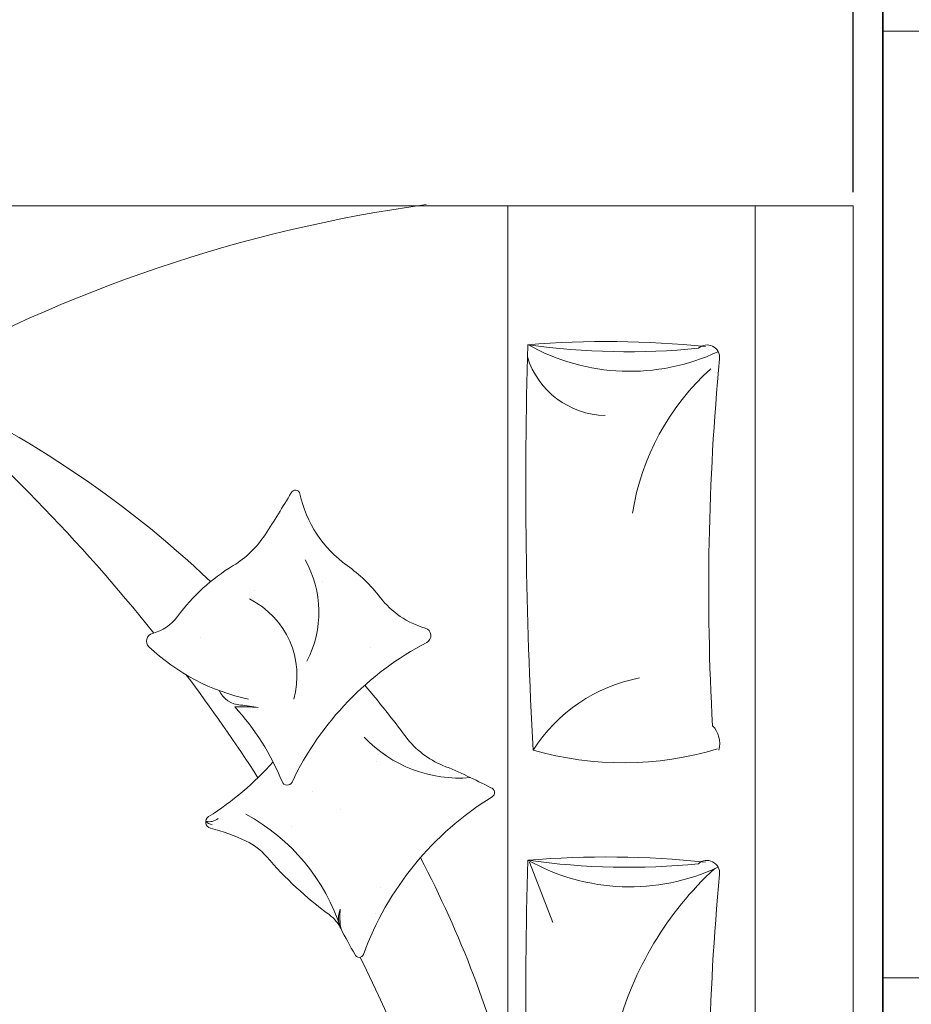
# Model space of a CAD drawing. Units: inches. Extents: x 3321 to 5237, y 11 to 1752.
# Tile 18 of 43: x 4413 to 4458, y 1230 to 1280. Entities that reach past the tile are written whole.
import ezdxf

# ---------------------------------------------------------------- set-up
doc = ezdxf.new("R2010")
doc.units = ezdxf.units.IN
for name, color, linetype, lineweight in [('A-ANNO-DIMS', 2, 'Continuous', 18), ('A-GLAZ', 5, 'Continuous', 18), ('A-WALL', 7, 'Continuous', 35), ('FUR', 42, 'Continuous', 18)]:
    doc.layers.add(name, color=color, linetype=linetype, lineweight=lineweight)
doc.styles.get("Standard").update_dxf_attribs({"font": 'arial.ttf'})
doc.dimstyles.new('ISO-25', dxfattribs={"dimtxt": 9, "dimasz": 2.5, "dimexe": 1.25, "dimexo": 0.625, "dimtad": 1, "dimdec": 1, "dimlunit": 3, "dimtxsty": 'Standard', "dimcen": 2.5, "dimclrd": 4, "dimclre": 4, "dimclrt": 256, "dimadec": 0, "dimazin": 0, "dimtfac": 1, "dimtdec": 1, "dimtmove": 0, "dimatfit": 3, "dimfxl": 1, "dimarcsym": 0})

# ---------------------------------------------------------------- blocks, each defined once
blk = doc.blocks.new('*X127')
at = {"color": 0}
for p, q in [((3155.9, 8182.9), (3155.9, 8182.9)), ((3147.8, 8143.4), (3147.8, 8143.4)), ((3283, 8049.6), (3283, 8049.6)), ((3209.5, 8023.9), (3209.5, 8023.9)), ((3251.6, 7997), (3251.6, 7997)), ((3154.1, 7950.7), (3154.1, 7950.7))]:
    blk.add_line(p, q, dxfattribs=at)
blk = doc.blocks.new('*X126')
at = {"color": 0}
for p, q in [((3155.9, 8182.9), (3155.9, 8182.9)), ((3139.8, 7939.7), (3139.8, 7939.7))]:
    blk.add_line(p, q, dxfattribs=at)
blk = doc.blocks.new('*X125')
at = {"color": 0}
for p, q in [((3155.9, 8182.9), (3155.9, 8182.9)), ((3139.8, 7939.7), (3139.8, 7939.7))]:
    blk.add_line(p, q, dxfattribs=at)
blk = doc.blocks.new('*X124')
at = {"color": 0}
for p, q in [((3163, 7776.2), (3163, 7776.2)), ((3422.2, 7761.3), (3422.2, 7761.3)), ((3244.3, 7698.6), (3244.3, 7698.6)), ((3340.3, 7689.4), (3340.3, 7689.4)), ((3236.2, 7675.7), (3236.2, 7675.7))]:
    blk.add_line(p, q, dxfattribs=at)
blk = doc.blocks.new('BED1')
for p, q in [((0, -1000), (0, 800)), ((150, 800), (150, -1000)), ((528, 800), (528, -1000)), ((150, -1000), (0, -1000)), ((150, -1000), (2063.5, -1000))]:
    blk.add_line(p, q)
for points in [[(205.5, 619.6, 0.267769), (215.1, 582.4, -0.037739), (204.3, 21.8, 0.684696), (236.7, 5.5, -0.060702), (497.2, 0.1, -0.046649), (225.9, 3.1, -1.318436)], [(497.2, 0.1, 0.021276), (489.2, 619.6, -0.206383), (326.6, 509.4, 0.237198)], [(211.8, 12.8, 0.143972), (361.6, 262.9, 1.292232)], [(886.4, -150, -0.069098), (985, -66.5, 0.658965), (982.1, -48.7, -0.049789), (927.4, -29, -0.103757), (896.6, -5.4, 0.055725), (800.9, 83.3, -0.11866), (782.7, 104.9, 0.016811), (761.6, 143.9, 0.70791), (748.3, 144, -0.16964), (551.9, -96.6, 0.664036), (554, -110.7, 0.023706), (627, -144.7, -0.134834), (683.2, -188, 0.012748), (746.3, -267.4)], [(969.1, -259.1, 0.263265), (936.3, -236.9, -0.026108), (909.2, -233.2, 0.027613), (945.1, -234.2, -0.089259), (872.7, -120, 0.662242), (857.6, -119.3, -0.162037), (651.8, -332.7, 0.676499), (654, -354.5, -0.160513), (722.9, -401.5, 0.07473), (773.5, -450.3, -0.187721), (845.5, -559.9, 0.70791), (858.8, -561.4, -0.010003), (898.6, -497.3, -0.113819), (947.3, -450.2, 0.099539), (1032.5, -372.4, -0.173425), (1070.9, -346.4, 0.589988), (1076.2, -326.1, 0.137312), (923.9, -245.9, 0.137312)], [(489.2, -168.2, 0.144019), (207.6, -169.9, 0.248643)], [(205.5, -168.2, 0.267769), (215.1, -205.4, -0.037739), (204.3, -766, 0.684696), (236.7, -782.3, -0.060702), (497.2, -787.7, -0.046649), (225.9, -784.7, -1.318436)], [(497.2, -787.7, 0.021276), (489.2, -168.2, -0.206383), (326.6, -278.4, 0.237198)], [(1446, -733.4, -0.095039), (652.8, -1001.7)]]:
    blk.add_lwpolyline(points, format="xyb")
blk.add_lwpolyline([(494.7, 3.1), (458.9, 95.3)])
for centre, radius, start, end in [((3208.8, 1363.3), 2739.4, 191.8679, 206.3247), ((2098.7, 754.7), 1625, 193.905, 207.8169), ((751.8, 88.7), 34.9, 336.8352, 27.7218), ((684.2, 86), 100.3, 353.675, 10.882), ((1074.1, 198.8), 306.1, 197.8602, 241.5122), ((341.4, -277.7), 318.5, 60.7125, 115.009), ((983.7, -79.5), 20.8, 73.7967, 130.4566), ((978.5, -68.6), 14.3, 39.7097, 85.9506), ((602.5, -324), 198.6, 43.2035, 95.0556), ((3208.8, 1363.3), 2739.4, 212.9314, 216.951), ((981.1, -281.8), 131.1, 164.0372, 243.4536), ((980, -379), 163.4, 152.6104, 209.361), ((3208.8, 1363.3), 2739.4, 218.6329, 229.9449), ((2098.7, 754.7), 1625, 226.5887, 246.3156), ((-34.4, -471.2), 376.5, 312.0118, 350.9635), ((375.7, -807.4), 128.2, 17.4073, 88.5129), ((341.4, -1065.5), 318.5, 60.7125, 115.009)]:
    blk.add_arc(centre, radius, start, end)
for name in ['*X126', '*X125', '*X127', '*X124']:
    blk.add_blockref(name, (-2425.3, -8101.4))
blk = doc.blocks.new('WIN-48IN-9IN-WALL')
for p, q in [((0, 0), (0, 9)), ((48, 0), (48, 9)), ((0, 5), (48, 5)), ((0, 4), (48, 4))]:
    blk.add_line(p, q)
blk = doc.blocks.new('*D195')
at = {"layer": 'A-ANNO-DIMS', "color": 4, "lineweight": -2, "transparency": 16777216}
for p, q in [((4369.073, 1271.165), (4369.073, 1284.663)), ((4454.896, 1271.165), (4454.896, 1284.663)), ((4452.396, 1283.413), (4371.573, 1283.413))]:
    blk.add_line(p, q, dxfattribs=at)
at = {"layer": 'A-ANNO-DIMS', "color": 4, "transparency": 16777216}
for points in [[(4371.573, 1283.83), (4371.573, 1282.997), (4369.073, 1283.413)], [(4452.396, 1283.83), (4452.396, 1282.997), (4454.896, 1283.413)]]:
    blk.add_solid(points, dxfattribs=at)
at = {"layer": 'Defpoints', "color": 0, "transparency": 16777216}
for p in [(4369.073, 1283.413), (4369.073, 1270.54), (4454.896, 1270.54)]:
    blk.add_point(p, dxfattribs=at)
at = {"layer": 'A-ANNO-DIMS', "transparency": 16777216, "insert": (4411.984, 1288.56), "char_height": 9, "attachment_point": 5}
blk.add_mtext('BED 7\'-2"', dxfattribs=at)

msp = doc.modelspace()

# ---------------------------------------------------------------- linework, layer by layer
at = {"layer": 'A-WALL'}
msp.add_line((4456.386, 1283.339), (4456.386, 1181.339), dxfattribs=at)

# ---------------------------------------------------------------- block references
at = {"layer": 'A-GLAZ', "rotation": 89.99999999999613}
msp.add_blockref('WIN-48IN-9IN-WALL', (4465.386, 1231.339), dxfattribs=at)
at = {"layer": 'FUR', "xscale": 0.0331718847221821, "yscale": 0.0331718847221821, "zscale": 0.0331718847221821, "rotation": 180}
msp.add_blockref('BED1', (4454.896, 1237.313), dxfattribs=at)

# ---------------------------------------------------------------- dimensions: what is measured, and where the dimension line sits
at = {"layer": 'A-ANNO-DIMS'}
dim = msp.add_linear_dim(base=(4369.073, 1283.413), p1=(4454.896, 1270.54), p2=(4369.073, 1270.54), angle=180, text='BED <>', dimstyle='ISO-25', override={"dimdec": 1, "dimlfac": 1, "dimrnd": 0, "dimzin": 1, "dimdsep": 46, "dimlunit": 4, "dimfrac": 2}, dxfattribs=at)
dim.commit()
dim.dimension.update_dxf_attribs({"geometry": '*D195', "text_midpoint": (4411.984, 1288.56)})

doc.saveas('drawing.dxf')
